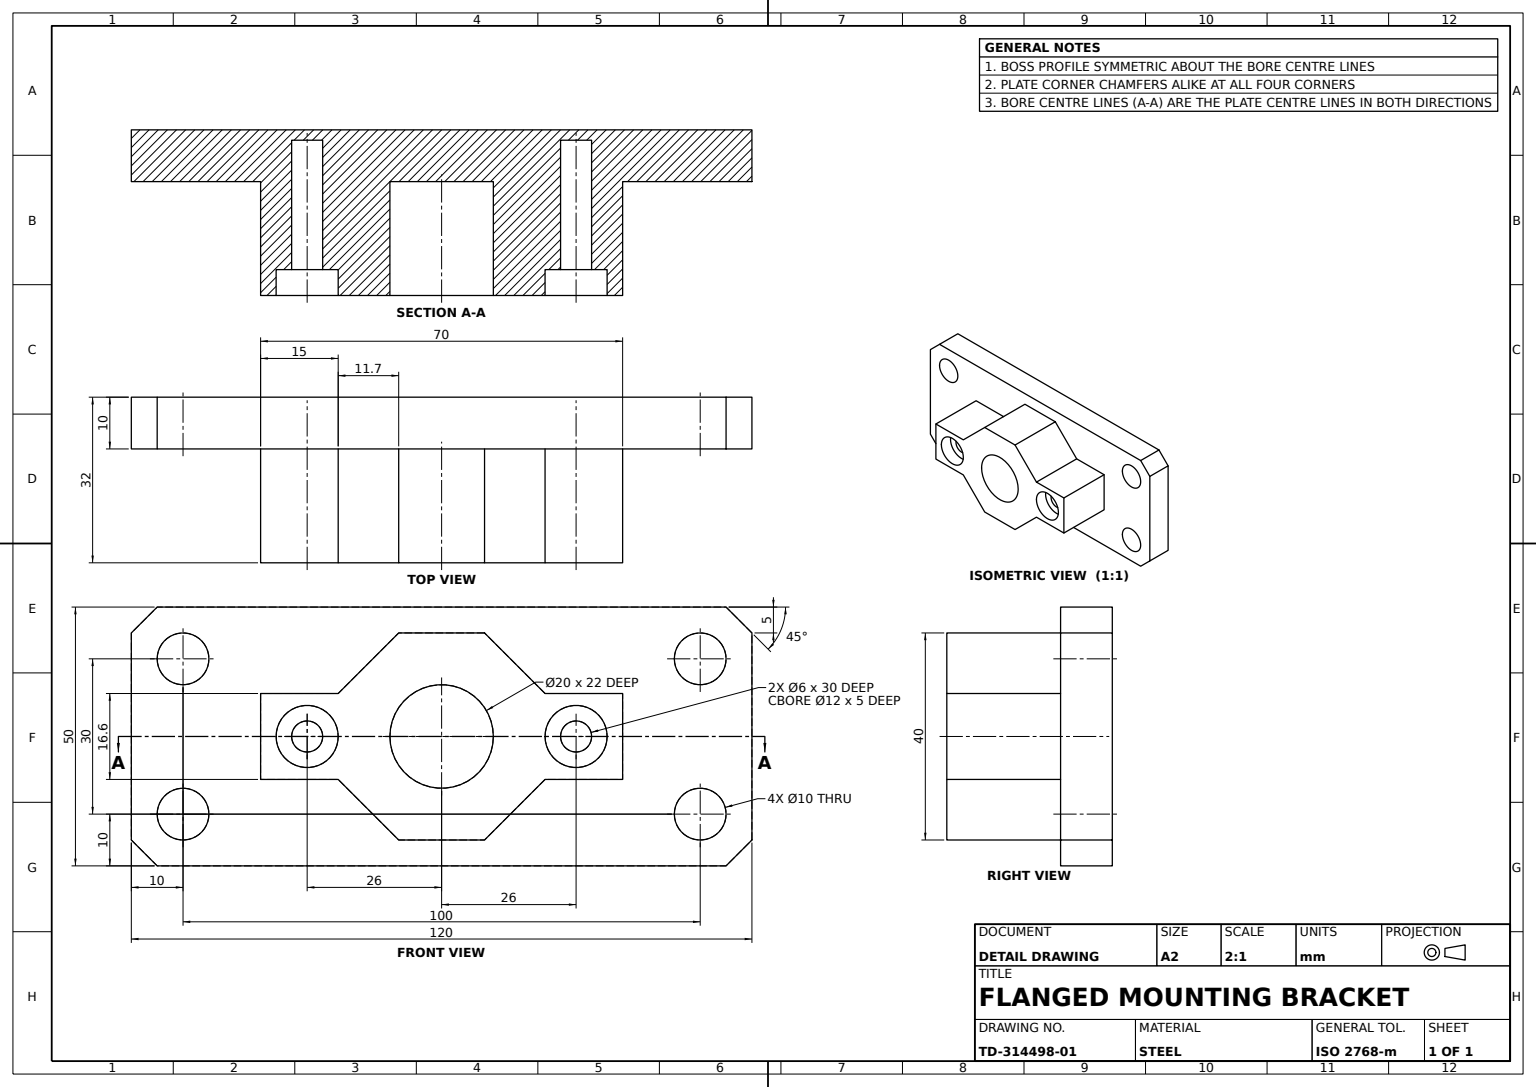
from build123d import *

# Parameters (mm, degrees)
BASE_PLATE_SKETCH_W        = 120
BASE_PLATE_SKETCH_H        = 50
BASE_PLATE_120X50X10_DEPTH = 10
CLAMP_BOSS_DEPTH           = 22
BORE_SKETCH_R              = 10
BORE_20_DEPTH              = 22
COUNTERBORE_SKETCH_R       = 6
COUNTERBORES_2X_12_DEPTH   = 5
BOLT_HOLE_SKETCH_R         = 3
BOLT_HOLES_2X_6_DEPTH      = 25
MOUNTING_HOLE_SKETCH_R     = 5
MOUNTING_HOLES_4X_10_DEPTH = 25
CORNER_CHAMFERS_5MM_SIZE   = 5


with BuildPart() as part:
    # Base Plate Sketch → Base Plate 120x50x10 (new body)
    with BuildSketch(Plane.XY):
        Rectangle(BASE_PLATE_SKETCH_W, BASE_PLATE_SKETCH_H)
    extrude(amount=BASE_PLATE_120X50X10_DEPTH)

    # Clamp Boss Sketch → Clamp Boss (add)
    with BuildSketch(Plane.XY.offset(10)):
        Polygon((20, 8.3), (35, 8.3), (35, -8.3), (20, -8.3), (8.3, -20), (-8.3, -20), (-20, -8.3), (-35, -8.3), (-35, 8.3), (-20, 8.3), (-8.3, 20), (8.3, 20), align=None)
    extrude(amount=CLAMP_BOSS_DEPTH)

    # Bore Sketch → Bore Ø20 (cut)
    with BuildSketch(Plane.XY.offset(32)):
        Circle(BORE_SKETCH_R)
    extrude(amount=-BORE_20_DEPTH, mode=Mode.SUBTRACT)

    # Counterbore Sketch → Counterbores 2xØ12 (cut)
    with BuildSketch(Plane.XY.offset(32)):
        with Locations((-26, 0)):
            Circle(COUNTERBORE_SKETCH_R)
        with Locations((26, 0)):
            Circle(COUNTERBORE_SKETCH_R)
    extrude(amount=-COUNTERBORES_2X_12_DEPTH, mode=Mode.SUBTRACT)

    # Bolt Hole Sketch → Bolt Holes 2xØ6 (cut)
    with BuildSketch(Plane.XY.offset(27)):
        with Locations((-26, 0)):
            Circle(BOLT_HOLE_SKETCH_R)
        with Locations((26, 0)):
            Circle(BOLT_HOLE_SKETCH_R)
    extrude(amount=-BOLT_HOLES_2X_6_DEPTH, mode=Mode.SUBTRACT)

    # Mounting Hole Sketch → Mounting Holes 4xØ10 (cut)
    with BuildSketch(Plane.XY.offset(10)):
        with Locations((50, 15)):
            Circle(MOUNTING_HOLE_SKETCH_R)
        with Locations((50, -15)):
            Circle(MOUNTING_HOLE_SKETCH_R)
        with Locations((-50, 15)):
            Circle(MOUNTING_HOLE_SKETCH_R)
        with Locations((-50, -15)):
            Circle(MOUNTING_HOLE_SKETCH_R)
    extrude(amount=-MOUNTING_HOLES_4X_10_DEPTH, mode=Mode.SUBTRACT)

    # Corner Chamfers 5mm
    corner_chamfers_5mm_edges = [part.edges().sort_by_distance(p)[0] for p in [
        (60, -25, 5),
        (-60, -25, 5),
        (-60, 25, 5),
        (60, 25, 5),
    ]]
    chamfer(corner_chamfers_5mm_edges, length=CORNER_CHAMFERS_5MM_SIZE)


solid = part.part
